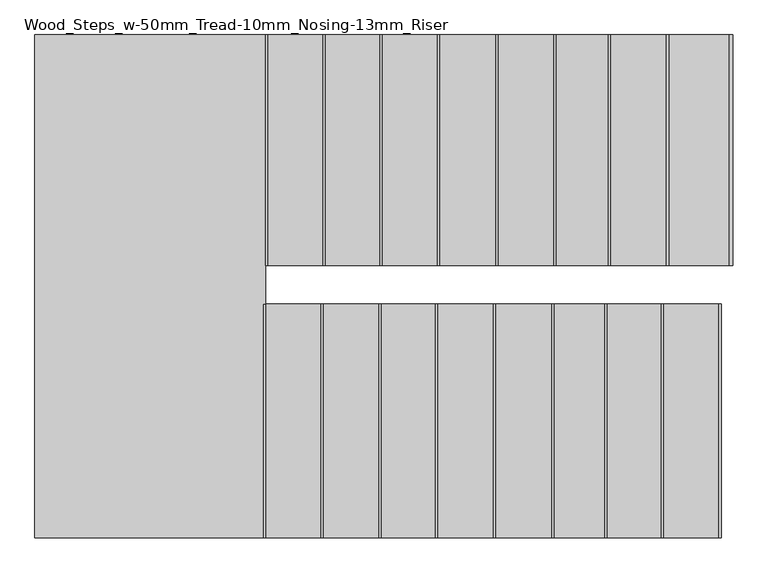
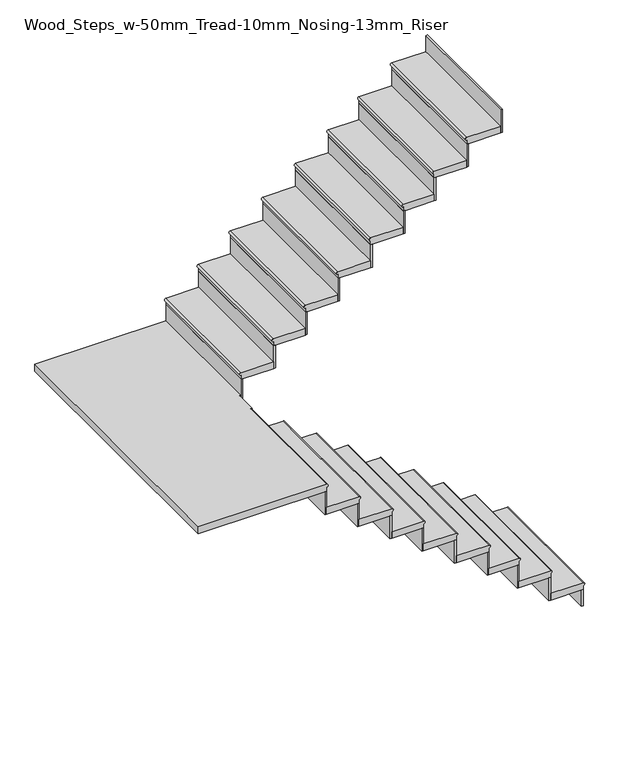
"""IFC4 building model written with IfcOpenShell, lengths in millimetres: stair flight geometry, Wood_Steps_w-50mm_Tread-10mm_Nosing-13mm_Riser."""

from ifc_helpers import new_model, si_unit, frame, origin, place, context, project, spatial, circle_curve, faceted_brep, source, transform, mapped, element, save
from ifc_brep_helpers import plane_surface, cylinder_surface, advanced_brep


def wood_steps_w_50mm_tread_10mm_nosing_13mm_riser_f1b6b8d3(model_context):
    return source(origin(), model_context, "Body", "SolidModel", [
        advanced_brep(
        [(3917.9747157, 6741.6853898, 149.3333333), (3917.9747157, 6741.6853898, 169.3333333), (3917.9747157, 5820.9272041, 169.3333333), (3917.9747157, 5820.9272041, 149.3333333), (3689.3747157, 5820.9272041, 169.3333333), (3689.3747157, 6741.6853898, 169.3333333), (3917.9747157, 5820.9272041, 119.3333333), (3689.3747157, 5820.9272041, 119.3333333), (3689.3747157, 6741.6853898, 119.3333333), (3917.9747157, 6741.6853898, 119.3333333)],
        [
            (0, 1, circle_curve(frame((3917.9747157, 6741.6853898, 159.3333333), z_axis=(0.0, -1.0, 0.0), x_axis=(-1.0, 0.0, 0.0)), 10.0)),
            (1, 2),
            (2, 3, circle_curve(frame((3917.9747157, 5820.9272041, 159.3333333), z_axis=(0.0, 1.0, 0.0), x_axis=(-1.0, 0.0, 0.0)), 10.0)),
            (3, 0),
            (4, 2),
            (1, 5),
            (5, 4),
            (6, 7),
            (7, 8),
            (8, 9),
            (9, 6),
            (4, 7),
            (6, 3),
            (9, 0),
            (8, 5),
        ],
        [
            cylinder_surface(frame((3917.9747157, 6741.6853898, 159.3333333), z_axis=(0.0, 1.0, 0.0), x_axis=(-1.0, 0.0, 0.0)), 10.0),
            plane_surface(frame((3927.9747157, 5820.9272041, 169.3333333), z_axis=(0.0, 0.0, 1.0), x_axis=(1.0, 0.0, 0.0))),
            plane_surface(frame((3927.9747157, 5820.9272041, 119.3333333), z_axis=(0.0, 0.0, -1.0), x_axis=(-1.0, 0.0, 0.0))),
            plane_surface(frame((3689.3747157, 5820.9272041, 169.3333333), z_axis=(0.0, -1.0, 0.0), x_axis=(0.0, 0.0, -1.0))),
            plane_surface(frame((3917.9747157, 5820.9272041, 169.3333333), z_axis=(1.0, 0.0, 0.0), x_axis=(0.0, 0.0, -1.0))),
            plane_surface(frame((3917.9747157, 6741.6853898, 169.3333333), z_axis=(0.0, 1.0, 0.0), x_axis=(0.0, 0.0, -1.0))),
            plane_surface(frame((3689.3747157, 6741.6853898, 169.3333333), z_axis=(-1.0, 0.0, 0.0), x_axis=(0.0, 0.0, -1.0))),
        ],
        [
            (0, [[1, 2, 3, 4]]),
            (1, [[5, -2, 6, 7]]),
            (2, [[8, 9, 10, 11]]),
            (3, [[-5, 12, -8, 13, -3]]),
            (4, [[-11, 14, -4, -13]]),
            (5, [[-6, -1, -14, -10, 15]]),
            (6, [[-7, -15, -9, -12]]),
        ],
    ),
        faceted_brep([(3917.9747157, 6741.6853898, 119.3333333), (3917.9747157, 6741.6853898, 0.0), (3905.4747157, 6741.6853898, 0.0), (3905.4747157, 6741.6853898, 119.3333333), (3917.9747157, 5820.9272041, 119.3333333), (3905.4747157, 5820.9272041, 119.3333333), (3905.4747157, 5820.9272041, 0.0), (3917.9747157, 5820.9272041, 0.0)], [[[0, 1, 2, 3]], [[4, 5, 6, 7]], [[1, 0, 4, 7]], [[2, 1, 7, 6]], [[3, 2, 6, 5]], [[0, 3, 5, 4]]]),
        faceted_brep([(3689.3747157, 6741.6853898, 288.6666667), (3689.3747157, 6741.6853898, 119.3333333), (3676.8747157, 6741.6853898, 119.3333333), (3676.8747157, 6741.6853898, 288.6666667), (3689.3747157, 5820.9272041, 288.6666667), (3676.8747157, 5820.9272041, 288.6666667), (3676.8747157, 5820.9272041, 119.3333333), (3689.3747157, 5820.9272041, 119.3333333)], [[[0, 1, 2, 3]], [[4, 5, 6, 7]], [[1, 0, 4, 7]], [[2, 1, 7, 6]], [[3, 2, 6, 5]], [[0, 3, 5, 4]]]),
        advanced_brep(
        [(3467.1247157, 5820.9272041, 338.6666667), (3689.3747157, 5820.9272041, 338.6666667), (3689.3747157, 6741.6853898, 338.6666667), (3467.1247157, 6741.6853898, 338.6666667), (3689.3747157, 5820.9272041, 288.6666667), (3467.1247157, 5820.9272041, 288.6666667), (3467.1247157, 6741.6853898, 288.6666667), (3689.3747157, 6741.6853898, 288.6666667), (3689.3747157, 5820.9272041, 318.6666667), (3689.3747157, 6741.6853898, 318.6666667)],
        [
            (0, 1),
            (1, 2),
            (2, 3),
            (3, 0),
            (4, 5),
            (5, 6),
            (6, 7),
            (7, 4),
            (0, 5),
            (4, 8),
            (8, 1, circle_curve(frame((3689.3747157, 5820.9272041, 328.6666667), z_axis=(0.0, -1.0, 0.0), x_axis=(-1.0, 0.0, 0.0)), 10.0)),
            (7, 9),
            (9, 8),
            (2, 9, circle_curve(frame((3689.3747157, 6741.6853898, 328.6666667), z_axis=(0.0, 1.0, 0.0), x_axis=(-1.0, 0.0, 0.0)), 10.0)),
            (6, 3),
        ],
        [
            plane_surface(frame((3927.9747157, 5820.9272041, 338.6666667), z_axis=(0.0, 0.0, 1.0), x_axis=(1.0, 0.0, 0.0))),
            plane_surface(frame((3927.9747157, 5820.9272041, 288.6666667), z_axis=(0.0, 0.0, -1.0), x_axis=(-1.0, 0.0, 0.0))),
            plane_surface(frame((3467.1247157, 5820.9272041, 338.6666667), z_axis=(0.0, -1.0, 0.0), x_axis=(0.0, 0.0, -1.0))),
            plane_surface(frame((3689.3747157, 5820.9272041, 338.6666667), z_axis=(1.0, 0.0, 0.0), x_axis=(0.0, 0.0, -1.0))),
            plane_surface(frame((3689.3747157, 6741.6853898, 338.6666667), z_axis=(0.0, 1.0, 0.0), x_axis=(0.0, 0.0, -1.0))),
            plane_surface(frame((3467.1247157, 6741.6853898, 338.6666667), z_axis=(-1.0, 0.0, 0.0), x_axis=(0.0, 0.0, -1.0))),
            cylinder_surface(frame((3689.3747157, 6741.6853898, 328.6666667), z_axis=(0.0, 1.0, 0.0), x_axis=(-1.0, 0.0, 0.0)), 10.0),
        ],
        [
            (0, [[1, 2, 3, 4]]),
            (1, [[5, 6, 7, 8]]),
            (2, [[-1, 9, -5, 10, 11]]),
            (3, [[-8, 12, 13, -10]]),
            (4, [[-3, 14, -12, -7, 15]]),
            (5, [[-4, -15, -6, -9]]),
            (6, [[-14, -2, -11, -13]]),
        ],
    ),
        faceted_brep([(3467.1247157, 6741.6853898, 458.0), (3467.1247157, 6741.6853898, 288.6666667), (3454.6247157, 6741.6853898, 288.6666667), (3454.6247157, 6741.6853898, 458.0), (3467.1247157, 5820.9272041, 458.0), (3454.6247157, 5820.9272041, 458.0), (3454.6247157, 5820.9272041, 288.6666667), (3467.1247157, 5820.9272041, 288.6666667)], [[[0, 1, 2, 3]], [[4, 5, 6, 7]], [[1, 0, 4, 7]], [[2, 1, 7, 6]], [[3, 2, 6, 5]], [[0, 3, 5, 4]]]),
        advanced_brep(
        [(3257.5747157, 5820.9272041, 508.0), (3467.1247157, 5820.9272041, 508.0), (3467.1247157, 6741.6853898, 508.0), (3257.5747157, 6741.6853898, 508.0), (3467.1247157, 5820.9272041, 458.0), (3257.5747157, 5820.9272041, 458.0), (3257.5747157, 6741.6853898, 458.0), (3467.1247157, 6741.6853898, 458.0), (3467.1247157, 5820.9272041, 488.0), (3467.1247157, 6741.6853898, 488.0)],
        [
            (0, 1),
            (1, 2),
            (2, 3),
            (3, 0),
            (4, 5),
            (5, 6),
            (6, 7),
            (7, 4),
            (0, 5),
            (4, 8),
            (8, 1, circle_curve(frame((3467.1247157, 5820.9272041, 498.0), z_axis=(0.0, -1.0, 0.0), x_axis=(-1.0, 0.0, 0.0)), 10.0)),
            (7, 9),
            (9, 8),
            (2, 9, circle_curve(frame((3467.1247157, 6741.6853898, 498.0), z_axis=(0.0, 1.0, 0.0), x_axis=(-1.0, 0.0, 0.0)), 10.0)),
            (6, 3),
        ],
        [
            plane_surface(frame((3927.9747157, 5820.9272041, 508.0), z_axis=(0.0, 0.0, 1.0), x_axis=(1.0, 0.0, 0.0))),
            plane_surface(frame((3927.9747157, 5820.9272041, 458.0), z_axis=(0.0, 0.0, -1.0), x_axis=(-1.0, 0.0, 0.0))),
            plane_surface(frame((3257.5747157, 5820.9272041, 508.0), z_axis=(0.0, -1.0, 0.0), x_axis=(0.0, 0.0, -1.0))),
            plane_surface(frame((3467.1247157, 5820.9272041, 508.0), z_axis=(1.0, 0.0, 0.0), x_axis=(0.0, 0.0, -1.0))),
            plane_surface(frame((3467.1247157, 6741.6853898, 508.0), z_axis=(0.0, 1.0, 0.0), x_axis=(0.0, 0.0, -1.0))),
            plane_surface(frame((3257.5747157, 6741.6853898, 508.0), z_axis=(-1.0, 0.0, 0.0), x_axis=(0.0, 0.0, -1.0))),
            cylinder_surface(frame((3467.1247157, 6741.6853898, 498.0), z_axis=(0.0, 1.0, 0.0), x_axis=(-1.0, 0.0, 0.0)), 10.0),
        ],
        [
            (0, [[1, 2, 3, 4]]),
            (1, [[5, 6, 7, 8]]),
            (2, [[-1, 9, -5, 10, 11]]),
            (3, [[-8, 12, 13, -10]]),
            (4, [[-3, 14, -12, -7, 15]]),
            (5, [[-4, -15, -6, -9]]),
            (6, [[-14, -2, -11, -13]]),
        ],
    ),
        faceted_brep([(3257.5747157, 6741.6853898, 627.3333333), (3257.5747157, 6741.6853898, 458.0), (3245.0747157, 6741.6853898, 458.0), (3245.0747157, 6741.6853898, 627.3333333), (3257.5747157, 5820.9272041, 627.3333333), (3245.0747157, 5820.9272041, 627.3333333), (3245.0747157, 5820.9272041, 458.0), (3257.5747157, 5820.9272041, 458.0)], [[[0, 1, 2, 3]], [[4, 5, 6, 7]], [[1, 0, 4, 7]], [[2, 1, 7, 6]], [[3, 2, 6, 5]], [[0, 3, 5, 4]]]),
        advanced_brep(
        [(3028.9747157, 5820.9272041, 677.3333333), (3257.5747157, 5820.9272041, 677.3333333), (3257.5747157, 6741.6853898, 677.3333333), (3028.9747157, 6741.6853898, 677.3333333), (3257.5747157, 5820.9272041, 627.3333333), (3028.9747157, 5820.9272041, 627.3333333), (3028.9747157, 6741.6853898, 627.3333333), (3257.5747157, 6741.6853898, 627.3333333), (3257.5747157, 5820.9272041, 657.3333333), (3257.5747157, 6741.6853898, 657.3333333)],
        [
            (0, 1),
            (1, 2),
            (2, 3),
            (3, 0),
            (4, 5),
            (5, 6),
            (6, 7),
            (7, 4),
            (0, 5),
            (4, 8),
            (8, 1, circle_curve(frame((3257.5747157, 5820.9272041, 667.3333333), z_axis=(0.0, -1.0, 0.0), x_axis=(-1.0, 0.0, 0.0)), 10.0)),
            (7, 9),
            (9, 8),
            (2, 9, circle_curve(frame((3257.5747157, 6741.6853898, 667.3333333), z_axis=(0.0, 1.0, 0.0), x_axis=(-1.0, 0.0, 0.0)), 10.0)),
            (6, 3),
        ],
        [
            plane_surface(frame((3927.9747157, 5820.9272041, 677.3333333), z_axis=(0.0, 0.0, 1.0), x_axis=(1.0, 0.0, 0.0))),
            plane_surface(frame((3927.9747157, 5820.9272041, 627.3333333), z_axis=(0.0, 0.0, -1.0), x_axis=(-1.0, 0.0, 0.0))),
            plane_surface(frame((3028.9747157, 5820.9272041, 677.3333333), z_axis=(0.0, -1.0, 0.0), x_axis=(0.0, 0.0, -1.0))),
            plane_surface(frame((3257.5747157, 5820.9272041, 677.3333333), z_axis=(1.0, 0.0, 0.0), x_axis=(0.0, 0.0, -1.0))),
            plane_surface(frame((3257.5747157, 6741.6853898, 677.3333333), z_axis=(0.0, 1.0, 0.0), x_axis=(0.0, 0.0, -1.0))),
            plane_surface(frame((3028.9747157, 6741.6853898, 677.3333333), z_axis=(-1.0, 0.0, 0.0), x_axis=(0.0, 0.0, -1.0))),
            cylinder_surface(frame((3257.5747157, 6741.6853898, 667.3333333), z_axis=(0.0, 1.0, 0.0), x_axis=(-1.0, 0.0, 0.0)), 10.0),
        ],
        [
            (0, [[1, 2, 3, 4]]),
            (1, [[5, 6, 7, 8]]),
            (2, [[-1, 9, -5, 10, 11]]),
            (3, [[-8, 12, 13, -10]]),
            (4, [[-3, 14, -12, -7, 15]]),
            (5, [[-4, -15, -6, -9]]),
            (6, [[-14, -2, -11, -13]]),
        ],
    ),
        faceted_brep([(3028.9747157, 6741.6853898, 796.6666667), (3028.9747157, 6741.6853898, 627.3333333), (3016.4747157, 6741.6853898, 627.3333333), (3016.4747157, 6741.6853898, 796.6666667), (3028.9747157, 5820.9272041, 796.6666667), (3016.4747157, 5820.9272041, 796.6666667), (3016.4747157, 5820.9272041, 627.3333333), (3028.9747157, 5820.9272041, 627.3333333)], [[[0, 1, 2, 3]], [[4, 5, 6, 7]], [[1, 0, 4, 7]], [[2, 1, 7, 6]], [[3, 2, 6, 5]], [[0, 3, 5, 4]]]),
        advanced_brep(
        [(2800.3747157, 5820.9272041, 846.6666667), (3028.9747157, 5820.9272041, 846.6666667), (3028.9747157, 6741.6853898, 846.6666667), (2800.3747157, 6741.6853898, 846.6666667), (3028.9747157, 5820.9272041, 796.6666667), (2800.3747157, 5820.9272041, 796.6666667), (2800.3747157, 6741.6853898, 796.6666667), (3028.9747157, 6741.6853898, 796.6666667), (3028.9747157, 5820.9272041, 826.6666667), (3028.9747157, 6741.6853898, 826.6666667)],
        [
            (0, 1),
            (1, 2),
            (2, 3),
            (3, 0),
            (4, 5),
            (5, 6),
            (6, 7),
            (7, 4),
            (0, 5),
            (4, 8),
            (8, 1, circle_curve(frame((3028.9747157, 5820.9272041, 836.6666667), z_axis=(0.0, -1.0, 0.0), x_axis=(-1.0, 0.0, 0.0)), 10.0)),
            (7, 9),
            (9, 8),
            (2, 9, circle_curve(frame((3028.9747157, 6741.6853898, 836.6666667), z_axis=(0.0, 1.0, 0.0), x_axis=(-1.0, 0.0, 0.0)), 10.0)),
            (6, 3),
        ],
        [
            plane_surface(frame((3699.3747157, 5820.9272041, 846.6666667), z_axis=(0.0, 0.0, 1.0), x_axis=(1.0, 0.0, 0.0))),
            plane_surface(frame((3699.3747157, 5820.9272041, 796.6666667), z_axis=(0.0, 0.0, -1.0), x_axis=(-1.0, 0.0, 0.0))),
            plane_surface(frame((2800.3747157, 5820.9272041, 846.6666667), z_axis=(0.0, -1.0, 0.0), x_axis=(0.0, 0.0, -1.0))),
            plane_surface(frame((3028.9747157, 5820.9272041, 846.6666667), z_axis=(1.0, 0.0, 0.0), x_axis=(0.0, 0.0, -1.0))),
            plane_surface(frame((3028.9747157, 6741.6853898, 846.6666667), z_axis=(0.0, 1.0, 0.0), x_axis=(0.0, 0.0, -1.0))),
            plane_surface(frame((2800.3747157, 6741.6853898, 846.6666667), z_axis=(-1.0, 0.0, 0.0), x_axis=(0.0, 0.0, -1.0))),
            cylinder_surface(frame((3028.9747157, 6741.6853898, 836.6666667), z_axis=(0.0, 1.0, 0.0), x_axis=(-1.0, 0.0, 0.0)), 10.0),
        ],
        [
            (0, [[1, 2, 3, 4]]),
            (1, [[5, 6, 7, 8]]),
            (2, [[-1, 9, -5, 10, 11]]),
            (3, [[-8, 12, 13, -10]]),
            (4, [[-3, 14, -12, -7, 15]]),
            (5, [[-4, -15, -6, -9]]),
            (6, [[-14, -2, -11, -13]]),
        ],
    ),
        faceted_brep([(2800.3747157, 6741.6853898, 966.0), (2800.3747157, 6741.6853898, 796.6666667), (2787.8747157, 6741.6853898, 796.6666667), (2787.8747157, 6741.6853898, 966.0), (2800.3747157, 5820.9272041, 966.0), (2787.8747157, 5820.9272041, 966.0), (2787.8747157, 5820.9272041, 796.6666667), (2800.3747157, 5820.9272041, 796.6666667)], [[[0, 1, 2, 3]], [[4, 5, 6, 7]], [[1, 0, 4, 7]], [[2, 1, 7, 6]], [[3, 2, 6, 5]], [[0, 3, 5, 4]]]),
        advanced_brep(
        [(2578.1247157, 5820.9272041, 1016.0), (2800.3747157, 5820.9272041, 1016.0), (2800.3747157, 6741.6853898, 1016.0), (2578.1247157, 6741.6853898, 1016.0), (2800.3747157, 5820.9272041, 966.0), (2578.1247157, 5820.9272041, 966.0), (2578.1247157, 6741.6853898, 966.0), (2800.3747157, 6741.6853898, 966.0), (2800.3747157, 5820.9272041, 996.0), (2800.3747157, 6741.6853898, 996.0)],
        [
            (0, 1),
            (1, 2),
            (2, 3),
            (3, 0),
            (4, 5),
            (5, 6),
            (6, 7),
            (7, 4),
            (0, 5),
            (4, 8),
            (8, 1, circle_curve(frame((2800.3747157, 5820.9272041, 1006.0), z_axis=(0.0, -1.0, 0.0), x_axis=(-1.0, 0.0, 0.0)), 10.0)),
            (7, 9),
            (9, 8),
            (2, 9, circle_curve(frame((2800.3747157, 6741.6853898, 1006.0), z_axis=(0.0, 1.0, 0.0), x_axis=(-1.0, 0.0, 0.0)), 10.0)),
            (6, 3),
        ],
        [
            plane_surface(frame((3927.9747157, 5820.9272041, 1016.0), z_axis=(0.0, 0.0, 1.0), x_axis=(1.0, 0.0, 0.0))),
            plane_surface(frame((3927.9747157, 5820.9272041, 966.0), z_axis=(0.0, 0.0, -1.0), x_axis=(-1.0, 0.0, 0.0))),
            plane_surface(frame((2578.1247157, 5820.9272041, 1016.0), z_axis=(0.0, -1.0, 0.0), x_axis=(0.0, 0.0, -1.0))),
            plane_surface(frame((2800.3747157, 5820.9272041, 1016.0), z_axis=(1.0, 0.0, 0.0), x_axis=(0.0, 0.0, -1.0))),
            plane_surface(frame((2800.3747157, 6741.6853898, 1016.0), z_axis=(0.0, 1.0, 0.0), x_axis=(0.0, 0.0, -1.0))),
            plane_surface(frame((2578.1247157, 6741.6853898, 1016.0), z_axis=(-1.0, 0.0, 0.0), x_axis=(0.0, 0.0, -1.0))),
            cylinder_surface(frame((2800.3747157, 6741.6853898, 1006.0), z_axis=(0.0, 1.0, 0.0), x_axis=(-1.0, 0.0, 0.0)), 10.0),
        ],
        [
            (0, [[1, 2, 3, 4]]),
            (1, [[5, 6, 7, 8]]),
            (2, [[-1, 9, -5, 10, 11]]),
            (3, [[-8, 12, 13, -10]]),
            (4, [[-3, 14, -12, -7, 15]]),
            (5, [[-4, -15, -6, -9]]),
            (6, [[-14, -2, -11, -13]]),
        ],
    ),
        faceted_brep([(2578.1247157, 6741.6853898, 1135.3333333), (2578.1247157, 6741.6853898, 966.0), (2565.6247157, 6741.6853898, 966.0), (2565.6247157, 6741.6853898, 1135.3333333), (2578.1247157, 5820.9272041, 1135.3333333), (2565.6247157, 5820.9272041, 1135.3333333), (2565.6247157, 5820.9272041, 966.0), (2578.1247157, 5820.9272041, 966.0)], [[[0, 1, 2, 3]], [[4, 5, 6, 7]], [[1, 0, 4, 7]], [[2, 1, 7, 6]], [[3, 2, 6, 5]], [[0, 3, 5, 4]]]),
        advanced_brep(
        [(2349.5247157, 5820.9272041, 1185.3333333), (2578.1247157, 5820.9272041, 1185.3333333), (2578.1247157, 6741.6853898, 1185.3333333), (2349.5247157, 6741.6853898, 1185.3333333), (2578.1247157, 5820.9272041, 1135.3333333), (2349.5247157, 5820.9272041, 1135.3333333), (2349.5247157, 6741.6853898, 1135.3333333), (2578.1247157, 6741.6853898, 1135.3333333), (2578.1247157, 5820.9272041, 1165.3333333), (2578.1247157, 6741.6853898, 1165.3333333)],
        [
            (0, 1),
            (1, 2),
            (2, 3),
            (3, 0),
            (4, 5),
            (5, 6),
            (6, 7),
            (7, 4),
            (0, 5),
            (4, 8),
            (8, 1, circle_curve(frame((2578.1247157, 5820.9272041, 1175.3333333), z_axis=(0.0, -1.0, 0.0), x_axis=(-1.0, 0.0, 0.0)), 10.0)),
            (7, 9),
            (9, 8),
            (2, 9, circle_curve(frame((2578.1247157, 6741.6853898, 1175.3333333), z_axis=(0.0, 1.0, 0.0), x_axis=(-1.0, 0.0, 0.0)), 10.0)),
            (6, 3),
        ],
        [
            plane_surface(frame((3927.9747157, 5820.9272041, 1185.3333333), z_axis=(0.0, 0.0, 1.0), x_axis=(1.0, 0.0, 0.0))),
            plane_surface(frame((3927.9747157, 5820.9272041, 1135.3333333), z_axis=(0.0, 0.0, -1.0), x_axis=(-1.0, 0.0, 0.0))),
            plane_surface(frame((2349.5247157, 5820.9272041, 1185.3333333), z_axis=(0.0, -1.0, 0.0), x_axis=(0.0, 0.0, -1.0))),
            plane_surface(frame((2578.1247157, 5820.9272041, 1185.3333333), z_axis=(1.0, 0.0, 0.0), x_axis=(0.0, 0.0, -1.0))),
            plane_surface(frame((2578.1247157, 6741.6853898, 1185.3333333), z_axis=(0.0, 1.0, 0.0), x_axis=(0.0, 0.0, -1.0))),
            plane_surface(frame((2349.5247157, 6741.6853898, 1185.3333333), z_axis=(-1.0, 0.0, 0.0), x_axis=(0.0, 0.0, -1.0))),
            cylinder_surface(frame((2578.1247157, 6741.6853898, 1175.3333333), z_axis=(0.0, 1.0, 0.0), x_axis=(-1.0, 0.0, 0.0)), 10.0),
        ],
        [
            (0, [[1, 2, 3, 4]]),
            (1, [[5, 6, 7, 8]]),
            (2, [[-1, 9, -5, 10, 11]]),
            (3, [[-8, 12, 13, -10]]),
            (4, [[-3, 14, -12, -7, 15]]),
            (5, [[-4, -15, -6, -9]]),
            (6, [[-14, -2, -11, -13]]),
        ],
    ),
        faceted_brep([(2349.5247157, 6741.6853898, 1304.6666667), (2349.5247157, 6741.6853898, 1135.3333333), (2337.0247157, 6741.6853898, 1135.3333333), (2337.0247157, 6741.6853898, 1304.6666667), (2349.5247157, 5820.9272041, 1304.6666667), (2337.0247157, 5820.9272041, 1304.6666667), (2337.0247157, 5820.9272041, 1135.3333333), (2349.5247157, 5820.9272041, 1135.3333333)], [[[0, 1, 2, 3]], [[4, 5, 6, 7]], [[1, 0, 4, 7]], [[2, 1, 7, 6]], [[3, 2, 6, 5]], [[0, 3, 5, 4]]]),
        advanced_brep(
        [(2121.8179225, 5820.9272041, 1354.6666667), (2349.5247157, 5820.9272041, 1354.6666667), (2349.5247157, 6741.6853898, 1354.6666667), (2121.8179225, 6741.6853898, 1354.6666667), (2349.5247157, 5820.9272041, 1304.6666667), (2121.8179225, 5820.9272041, 1304.6666667), (2121.8179225, 6741.6853898, 1304.6666667), (2349.5247157, 6741.6853898, 1304.6666667), (2349.5247157, 5820.9272041, 1334.6666667), (2349.5247157, 6741.6853898, 1334.6666667)],
        [
            (0, 1),
            (1, 2),
            (2, 3),
            (3, 0),
            (4, 5),
            (5, 6),
            (6, 7),
            (7, 4),
            (0, 5),
            (4, 8),
            (8, 1, circle_curve(frame((2349.5247157, 5820.9272041, 1344.6666667), z_axis=(0.0, -1.0, 0.0), x_axis=(-1.0, 0.0, 0.0)), 10.0)),
            (7, 9),
            (9, 8),
            (2, 9, circle_curve(frame((2349.5247157, 6741.6853898, 1344.6666667), z_axis=(0.0, 1.0, 0.0), x_axis=(-1.0, 0.0, 0.0)), 10.0)),
            (6, 3),
        ],
        [
            plane_surface(frame((3927.9747157, 5820.9272041, 1354.6666667), z_axis=(0.0, 0.0, 1.0), x_axis=(1.0, 0.0, 0.0))),
            plane_surface(frame((3927.9747157, 5820.9272041, 1304.6666667), z_axis=(0.0, 0.0, -1.0), x_axis=(-1.0, 0.0, 0.0))),
            plane_surface(frame((2121.8179225, 5820.9272041, 1354.6666667), z_axis=(0.0, -1.0, 0.0), x_axis=(0.0, 0.0, -1.0))),
            plane_surface(frame((2349.5247157, 5820.9272041, 1354.6666667), z_axis=(1.0, 0.0, 0.0), x_axis=(0.0, 0.0, -1.0))),
            plane_surface(frame((2349.5247157, 6741.6853898, 1354.6666667), z_axis=(0.0, 1.0, 0.0), x_axis=(0.0, 0.0, -1.0))),
            plane_surface(frame((2121.8179225, 6741.6853898, 1354.6666667), z_axis=(-1.0, 0.0, 0.0), x_axis=(0.0, 0.0, -1.0))),
            cylinder_surface(frame((2349.5247157, 6741.6853898, 1344.6666667), z_axis=(0.0, 1.0, 0.0), x_axis=(-1.0, 0.0, 0.0)), 10.0),
        ],
        [
            (0, [[1, 2, 3, 4]]),
            (1, [[5, 6, 7, 8]]),
            (2, [[-1, 9, -5, 10, 11]]),
            (3, [[-8, 12, 13, -10]]),
            (4, [[-3, 14, -12, -7, 15]]),
            (5, [[-4, -15, -6, -9]]),
            (6, [[-14, -2, -11, -13]]),
        ],
    ),
        faceted_brep([(2121.8179225, 6741.6853898, 1474.0), (2121.8179225, 6741.6853898, 1304.6666667), (2109.3179225, 6741.6853898, 1304.6666667), (2109.3179225, 6741.6853898, 1474.0), (2121.8179225, 5820.9272041, 1474.0), (2109.3179225, 5820.9272041, 1474.0), (2109.3179225, 5820.9272041, 1304.6666667), (2121.8179225, 5820.9272041, 1304.6666667)], [[[0, 1, 2, 3]], [[4, 5, 6, 7]], [[1, 0, 4, 7]], [[2, 1, 7, 6]], [[3, 2, 6, 5]], [[0, 3, 5, 4]]]),
        advanced_brep(
        [(2141.8179225, 7802.1353898, 1524.0), (1223.7679225, 7802.1353898, 1524.0), (1223.7679225, 5820.9272041, 1524.0), (2121.8179225, 5820.9272041, 1524.0), (2121.8179225, 6741.6853898, 1524.0), (2131.8179225, 6741.6853898, 1524.0), (2131.8179225, 6894.0853898, 1524.0), (2141.8179225, 6894.0853898, 1524.0), (1223.7679225, 7802.1353898, 1474.0), (2141.8179225, 7802.1353898, 1474.0), (2141.8179225, 6894.0853898, 1474.0), (2131.8179225, 6894.0853898, 1474.0), (2131.8179225, 6741.6853898, 1474.0), (2121.8179225, 6741.6853898, 1474.0), (2121.8179225, 5820.9272041, 1474.0), (1223.7679225, 5820.9272041, 1474.0), (2121.8179225, 5820.9272041, 1504.0), (2121.8179225, 6741.6853898, 1504.0), (2131.8179225, 6741.6853898, 1514.0)],
        [
            (0, 1),
            (1, 2),
            (2, 3),
            (3, 4),
            (4, 5),
            (5, 6),
            (6, 7),
            (7, 0),
            (8, 9),
            (9, 10),
            (10, 11),
            (11, 12),
            (12, 13),
            (13, 14),
            (14, 15),
            (15, 8),
            (0, 9),
            (8, 1),
            (15, 2),
            (14, 16),
            (16, 3, circle_curve(frame((2121.8179225, 5820.9272041, 1514.0), z_axis=(0.0, -1.0, 0.0), x_axis=(-1.0, 0.0, 0.0)), 10.0)),
            (13, 17),
            (17, 16),
            (4, 18, circle_curve(frame((2121.8179225, 6741.6853898, 1514.0), z_axis=(0.0, 1.0, 0.0), x_axis=(-1.0, 0.0, 0.0)), 10.0)),
            (18, 5),
            (12, 18),
            (18, 17, circle_curve(frame((2121.8179225, 6741.6853898, 1514.0), z_axis=(0.0, 1.0, 0.0), x_axis=(-1.0, 0.0, 0.0)), 10.0)),
            (11, 6),
            (10, 7),
        ],
        [
            plane_surface(frame((1223.7679225, 7802.1353898, 1524.0), z_axis=(0.0, 0.0, 1.0), x_axis=(-1.0, 0.0, 0.0))),
            plane_surface(frame((1223.7679225, 7802.1353898, 1474.0), z_axis=(0.0, 0.0, -1.0), x_axis=(1.0, 0.0, 0.0))),
            plane_surface(frame((2141.8179225, 7802.1353898, 1524.0), z_axis=(0.0, 1.0, 0.0), x_axis=(0.0, 0.0, -1.0))),
            plane_surface(frame((1223.7679225, 7802.1353898, 1524.0), z_axis=(-1.0, 0.0, 0.0), x_axis=(0.0, 0.0, -1.0))),
            plane_surface(frame((1223.7679225, 5820.9272041, 1524.0), z_axis=(0.0, -1.0, 0.0), x_axis=(0.0, 0.0, -1.0))),
            plane_surface(frame((2121.8179225, 5820.9272041, 1524.0), z_axis=(1.0, 0.0, 0.0), x_axis=(0.0, 0.0, -1.0))),
            plane_surface(frame((2121.8179225, 6741.6853898, 1524.0), z_axis=(0.0, -1.0, 0.0), x_axis=(0.0, 0.0, -1.0))),
            plane_surface(frame((2131.8179225, 6741.6853898, 1524.0), z_axis=(1.0, 0.0, 0.0), x_axis=(0.0, 0.0, -1.0))),
            plane_surface(frame((2131.8179225, 6894.0853898, 1524.0), z_axis=(0.0, -1.0, 0.0), x_axis=(0.0, 0.0, -1.0))),
            plane_surface(frame((2141.8179225, 6894.0853898, 1524.0), z_axis=(1.0, 0.0, 0.0), x_axis=(0.0, 0.0, -1.0))),
            cylinder_surface(frame((2121.8179225, 6741.6853898, 1514.0), z_axis=(0.0, 1.0, 0.0), x_axis=(-1.0, 0.0, 0.0)), 10.0),
        ],
        [
            (0, [[1, 2, 3, 4, 5, 6, 7, 8]]),
            (1, [[9, 10, 11, 12, 13, 14, 15, 16]]),
            (2, [[-1, 17, -9, 18]]),
            (3, [[-2, -18, -16, 19]]),
            (4, [[-3, -19, -15, 20, 21]]),
            (5, [[-14, 22, 23, -20]]),
            (6, [[-5, 24, 25]]),
            (6, [[-13, 26, 27, -22]]),
            (7, [[-6, -25, -26, -12, 28]]),
            (8, [[-7, -28, -11, 29]]),
            (9, [[-8, -29, -10, -17]]),
            (10, [[-21, -23, -27, -24, -4]]),
        ],
    ),
        faceted_brep([(2141.8179225, 6894.0853898, 1643.3333333), (2141.8179225, 6894.0853898, 1474.0), (2154.3179225, 6894.0853898, 1474.0), (2154.3179225, 6894.0853898, 1643.3333333), (2141.8179225, 7802.1353898, 1643.3333333), (2154.3179225, 7802.1353898, 1643.3333333), (2154.3179225, 7802.1353898, 1474.0), (2141.8179225, 7802.1353898, 1474.0)], [[[0, 1, 2, 3]], [[4, 5, 6, 7]], [[1, 0, 4, 7]], [[2, 1, 7, 6]], [[3, 2, 6, 5]], [[0, 3, 5, 4]]]),
        advanced_brep(
        [(2369.5247157, 7802.1353898, 1693.3333333), (2141.8179225, 7802.1353898, 1693.3333333), (2141.8179225, 6894.0853898, 1693.3333333), (2369.5247157, 6894.0853898, 1693.3333333), (2141.8179225, 7802.1353898, 1643.3333333), (2369.5247157, 7802.1353898, 1643.3333333), (2369.5247157, 6894.0853898, 1643.3333333), (2141.8179225, 6894.0853898, 1643.3333333), (2141.8179225, 7802.1353898, 1673.3333333), (2141.8179225, 6894.0853898, 1673.3333333)],
        [
            (0, 1),
            (1, 2),
            (2, 3),
            (3, 0),
            (4, 5),
            (5, 6),
            (6, 7),
            (7, 4),
            (0, 5),
            (4, 8),
            (8, 1, circle_curve(frame((2141.8179225, 7802.1353898, 1683.3333333), z_axis=(0.0, 1.0, 0.0), x_axis=(1.0, 0.0, 0.0)), 10.0)),
            (7, 9),
            (9, 8),
            (2, 9, circle_curve(frame((2141.8179225, 6894.0853898, 1683.3333333), z_axis=(0.0, -1.0, 0.0), x_axis=(1.0, 0.0, 0.0)), 10.0)),
            (6, 3),
        ],
        [
            plane_surface(frame((1223.7679225, 7802.1353898, 1693.3333333), z_axis=(0.0, 0.0, 1.0), x_axis=(-1.0, 0.0, 0.0))),
            plane_surface(frame((1223.7679225, 7802.1353898, 1643.3333333), z_axis=(0.0, 0.0, -1.0), x_axis=(1.0, 0.0, 0.0))),
            plane_surface(frame((2369.5247157, 7802.1353898, 1693.3333333), z_axis=(0.0, 1.0, 0.0), x_axis=(0.0, 0.0, -1.0))),
            plane_surface(frame((2141.8179225, 7802.1353898, 1693.3333333), z_axis=(-1.0, 0.0, 0.0), x_axis=(0.0, 0.0, -1.0))),
            plane_surface(frame((2141.8179225, 6894.0853898, 1693.3333333), z_axis=(0.0, -1.0, 0.0), x_axis=(0.0, 0.0, -1.0))),
            plane_surface(frame((2369.5247157, 6894.0853898, 1693.3333333), z_axis=(1.0, 0.0, 0.0), x_axis=(0.0, 0.0, -1.0))),
            cylinder_surface(frame((2141.8179225, 6894.0853898, 1683.3333333), z_axis=(0.0, -1.0, 0.0), x_axis=(1.0, 0.0, 0.0)), 10.0),
        ],
        [
            (0, [[1, 2, 3, 4]]),
            (1, [[5, 6, 7, 8]]),
            (2, [[-1, 9, -5, 10, 11]]),
            (3, [[-8, 12, 13, -10]]),
            (4, [[-3, 14, -12, -7, 15]]),
            (5, [[-4, -15, -6, -9]]),
            (6, [[-14, -2, -11, -13]]),
        ],
    ),
        faceted_brep([(2369.5247157, 6894.0853898, 1812.6666667), (2369.5247157, 6894.0853898, 1643.3333333), (2382.0247157, 6894.0853898, 1643.3333333), (2382.0247157, 6894.0853898, 1812.6666667), (2369.5247157, 7802.1353898, 1812.6666667), (2382.0247157, 7802.1353898, 1812.6666667), (2382.0247157, 7802.1353898, 1643.3333333), (2369.5247157, 7802.1353898, 1643.3333333)], [[[0, 1, 2, 3]], [[4, 5, 6, 7]], [[1, 0, 4, 7]], [[2, 1, 7, 6]], [[3, 2, 6, 5]], [[0, 3, 5, 4]]]),
        advanced_brep(
        [(2592.6679225, 7802.1353898, 1862.6666667), (2369.5247157, 7802.1353898, 1862.6666667), (2369.5247157, 6894.0853898, 1862.6666667), (2592.6679225, 6894.0853898, 1862.6666667), (2369.5247157, 7802.1353898, 1812.6666667), (2592.6679225, 7802.1353898, 1812.6666667), (2592.6679225, 6894.0853898, 1812.6666667), (2369.5247157, 6894.0853898, 1812.6666667), (2369.5247157, 7802.1353898, 1842.6666667), (2369.5247157, 6894.0853898, 1842.6666667)],
        [
            (0, 1),
            (1, 2),
            (2, 3),
            (3, 0),
            (4, 5),
            (5, 6),
            (6, 7),
            (7, 4),
            (0, 5),
            (4, 8),
            (8, 1, circle_curve(frame((2369.5247157, 7802.1353898, 1852.6666667), z_axis=(0.0, 1.0, 0.0), x_axis=(1.0, 0.0, 0.0)), 10.0)),
            (7, 9),
            (9, 8),
            (2, 9, circle_curve(frame((2369.5247157, 6894.0853898, 1852.6666667), z_axis=(0.0, -1.0, 0.0), x_axis=(1.0, 0.0, 0.0)), 10.0)),
            (6, 3),
        ],
        [
            plane_surface(frame((1223.7679225, 7802.1353898, 1862.6666667), z_axis=(0.0, 0.0, 1.0), x_axis=(-1.0, 0.0, 0.0))),
            plane_surface(frame((1223.7679225, 7802.1353898, 1812.6666667), z_axis=(0.0, 0.0, -1.0), x_axis=(1.0, 0.0, 0.0))),
            plane_surface(frame((2592.6679225, 7802.1353898, 1862.6666667), z_axis=(0.0, 1.0, 0.0), x_axis=(0.0, 0.0, -1.0))),
            plane_surface(frame((2369.5247157, 7802.1353898, 1862.6666667), z_axis=(-1.0, 0.0, 0.0), x_axis=(0.0, 0.0, -1.0))),
            plane_surface(frame((2369.5247157, 6894.0853898, 1862.6666667), z_axis=(0.0, -1.0, 0.0), x_axis=(0.0, 0.0, -1.0))),
            plane_surface(frame((2592.6679225, 6894.0853898, 1862.6666667), z_axis=(1.0, 0.0, 0.0), x_axis=(0.0, 0.0, -1.0))),
            cylinder_surface(frame((2369.5247157, 6894.0853898, 1852.6666667), z_axis=(0.0, -1.0, 0.0), x_axis=(1.0, 0.0, 0.0)), 10.0),
        ],
        [
            (0, [[1, 2, 3, 4]]),
            (1, [[5, 6, 7, 8]]),
            (2, [[-1, 9, -5, 10, 11]]),
            (3, [[-8, 12, 13, -10]]),
            (4, [[-3, 14, -12, -7, 15]]),
            (5, [[-4, -15, -6, -9]]),
            (6, [[-14, -2, -11, -13]]),
        ],
    ),
        faceted_brep([(2592.6679225, 6894.0853898, 1982.0), (2592.6679225, 6894.0853898, 1812.6666667), (2605.1679225, 6894.0853898, 1812.6666667), (2605.1679225, 6894.0853898, 1982.0), (2592.6679225, 7802.1353898, 1982.0), (2605.1679225, 7802.1353898, 1982.0), (2605.1679225, 7802.1353898, 1812.6666667), (2592.6679225, 7802.1353898, 1812.6666667)], [[[0, 1, 2, 3]], [[4, 5, 6, 7]], [[1, 0, 4, 7]], [[2, 1, 7, 6]], [[3, 2, 6, 5]], [[0, 3, 5, 4]]]),
        advanced_brep(
        [(2820.3747157, 7802.1353898, 2032.0), (2592.6679225, 7802.1353898, 2032.0), (2592.6679225, 6894.0853898, 2032.0), (2820.3747157, 6894.0853898, 2032.0), (2592.6679225, 7802.1353898, 1982.0), (2820.3747157, 7802.1353898, 1982.0), (2820.3747157, 6894.0853898, 1982.0), (2592.6679225, 6894.0853898, 1982.0), (2592.6679225, 7802.1353898, 2012.0), (2592.6679225, 6894.0853898, 2012.0)],
        [
            (0, 1),
            (1, 2),
            (2, 3),
            (3, 0),
            (4, 5),
            (5, 6),
            (6, 7),
            (7, 4),
            (0, 5),
            (4, 8),
            (8, 1, circle_curve(frame((2592.6679225, 7802.1353898, 2022.0), z_axis=(0.0, 1.0, 0.0), x_axis=(1.0, 0.0, 0.0)), 10.0)),
            (7, 9),
            (9, 8),
            (2, 9, circle_curve(frame((2592.6679225, 6894.0853898, 2022.0), z_axis=(0.0, -1.0, 0.0), x_axis=(1.0, 0.0, 0.0)), 10.0)),
            (6, 3),
        ],
        [
            plane_surface(frame((1223.7679225, 7802.1353898, 2032.0), z_axis=(0.0, 0.0, 1.0), x_axis=(-1.0, 0.0, 0.0))),
            plane_surface(frame((1223.7679225, 7802.1353898, 1982.0), z_axis=(0.0, 0.0, -1.0), x_axis=(1.0, 0.0, 0.0))),
            plane_surface(frame((2820.3747157, 7802.1353898, 2032.0), z_axis=(0.0, 1.0, 0.0), x_axis=(0.0, 0.0, -1.0))),
            plane_surface(frame((2592.6679225, 7802.1353898, 2032.0), z_axis=(-1.0, 0.0, 0.0), x_axis=(0.0, 0.0, -1.0))),
            plane_surface(frame((2592.6679225, 6894.0853898, 2032.0), z_axis=(0.0, -1.0, 0.0), x_axis=(0.0, 0.0, -1.0))),
            plane_surface(frame((2820.3747157, 6894.0853898, 2032.0), z_axis=(1.0, 0.0, 0.0), x_axis=(0.0, 0.0, -1.0))),
            cylinder_surface(frame((2592.6679225, 6894.0853898, 2022.0), z_axis=(0.0, -1.0, 0.0), x_axis=(1.0, 0.0, 0.0)), 10.0),
        ],
        [
            (0, [[1, 2, 3, 4]]),
            (1, [[5, 6, 7, 8]]),
            (2, [[-1, 9, -5, 10, 11]]),
            (3, [[-8, 12, 13, -10]]),
            (4, [[-3, 14, -12, -7, 15]]),
            (5, [[-4, -15, -6, -9]]),
            (6, [[-14, -2, -11, -13]]),
        ],
    ),
        faceted_brep([(2820.3747157, 6894.0853898, 2151.3333333), (2820.3747157, 6894.0853898, 1982.0), (2832.8747157, 6894.0853898, 1982.0), (2832.8747157, 6894.0853898, 2151.3333333), (2820.3747157, 7802.1353898, 2151.3333333), (2832.8747157, 7802.1353898, 2151.3333333), (2832.8747157, 7802.1353898, 1982.0), (2820.3747157, 7802.1353898, 1982.0)], [[[0, 1, 2, 3]], [[4, 5, 6, 7]], [[1, 0, 4, 7]], [[2, 1, 7, 6]], [[3, 2, 6, 5]], [[0, 3, 5, 4]]]),
        advanced_brep(
        [(3048.9747157, 7802.1353898, 2201.3333333), (2820.3747157, 7802.1353898, 2201.3333333), (2820.3747157, 6894.0853898, 2201.3333333), (3048.9747157, 6894.0853898, 2201.3333333), (2820.3747157, 7802.1353898, 2151.3333333), (3048.9747157, 7802.1353898, 2151.3333333), (3048.9747157, 6894.0853898, 2151.3333333), (2820.3747157, 6894.0853898, 2151.3333333), (2820.3747157, 7802.1353898, 2181.3333333), (2820.3747157, 6894.0853898, 2181.3333333)],
        [
            (0, 1),
            (1, 2),
            (2, 3),
            (3, 0),
            (4, 5),
            (5, 6),
            (6, 7),
            (7, 4),
            (0, 5),
            (4, 8),
            (8, 1, circle_curve(frame((2820.3747157, 7802.1353898, 2191.3333333), z_axis=(0.0, 1.0, 0.0), x_axis=(1.0, 0.0, 0.0)), 10.0)),
            (7, 9),
            (9, 8),
            (2, 9, circle_curve(frame((2820.3747157, 6894.0853898, 2191.3333333), z_axis=(0.0, -1.0, 0.0), x_axis=(1.0, 0.0, 0.0)), 10.0)),
            (6, 3),
        ],
        [
            plane_surface(frame((1223.7679225, 7802.1353898, 2201.3333333), z_axis=(0.0, 0.0, 1.0), x_axis=(-1.0, 0.0, 0.0))),
            plane_surface(frame((1223.7679225, 7802.1353898, 2151.3333333), z_axis=(0.0, 0.0, -1.0), x_axis=(1.0, 0.0, 0.0))),
            plane_surface(frame((3048.9747157, 7802.1353898, 2201.3333333), z_axis=(0.0, 1.0, 0.0), x_axis=(0.0, 0.0, -1.0))),
            plane_surface(frame((2820.3747157, 7802.1353898, 2201.3333333), z_axis=(-1.0, 0.0, 0.0), x_axis=(0.0, 0.0, -1.0))),
            plane_surface(frame((2820.3747157, 6894.0853898, 2201.3333333), z_axis=(0.0, -1.0, 0.0), x_axis=(0.0, 0.0, -1.0))),
            plane_surface(frame((3048.9747157, 6894.0853898, 2201.3333333), z_axis=(1.0, 0.0, 0.0), x_axis=(0.0, 0.0, -1.0))),
            cylinder_surface(frame((2820.3747157, 6894.0853898, 2191.3333333), z_axis=(0.0, -1.0, 0.0), x_axis=(1.0, 0.0, 0.0)), 10.0),
        ],
        [
            (0, [[1, 2, 3, 4]]),
            (1, [[5, 6, 7, 8]]),
            (2, [[-1, 9, -5, 10, 11]]),
            (3, [[-8, 12, 13, -10]]),
            (4, [[-3, 14, -12, -7, 15]]),
            (5, [[-4, -15, -6, -9]]),
            (6, [[-14, -2, -11, -13]]),
        ],
    ),
        faceted_brep([(3048.9747157, 6894.0853898, 2320.6666667), (3048.9747157, 6894.0853898, 2151.3333333), (3061.4747157, 6894.0853898, 2151.3333333), (3061.4747157, 6894.0853898, 2320.6666667), (3048.9747157, 7802.1353898, 2320.6666667), (3061.4747157, 7802.1353898, 2320.6666667), (3061.4747157, 7802.1353898, 2151.3333333), (3048.9747157, 7802.1353898, 2151.3333333)], [[[0, 1, 2, 3]], [[4, 5, 6, 7]], [[1, 0, 4, 7]], [[2, 1, 7, 6]], [[3, 2, 6, 5]], [[0, 3, 5, 4]]]),
        advanced_brep(
        [(3277.5747157, 7802.1353898, 2370.6666667), (3048.9747157, 7802.1353898, 2370.6666667), (3048.9747157, 6894.0853898, 2370.6666667), (3277.5747157, 6894.0853898, 2370.6666667), (3048.9747157, 7802.1353898, 2320.6666667), (3277.5747157, 7802.1353898, 2320.6666667), (3277.5747157, 6894.0853898, 2320.6666667), (3048.9747157, 6894.0853898, 2320.6666667), (3048.9747157, 7802.1353898, 2350.6666667), (3048.9747157, 6894.0853898, 2350.6666667)],
        [
            (0, 1),
            (1, 2),
            (2, 3),
            (3, 0),
            (4, 5),
            (5, 6),
            (6, 7),
            (7, 4),
            (0, 5),
            (4, 8),
            (8, 1, circle_curve(frame((3048.9747157, 7802.1353898, 2360.6666667), z_axis=(0.0, 1.0, 0.0), x_axis=(1.0, 0.0, 0.0)), 10.0)),
            (7, 9),
            (9, 8),
            (2, 9, circle_curve(frame((3048.9747157, 6894.0853898, 2360.6666667), z_axis=(0.0, -1.0, 0.0), x_axis=(1.0, 0.0, 0.0)), 10.0)),
            (6, 3),
        ],
        [
            plane_surface(frame((1452.3679225, 7802.1353898, 2370.6666667), z_axis=(0.0, 0.0, 1.0), x_axis=(-1.0, 0.0, 0.0))),
            plane_surface(frame((1452.3679225, 7802.1353898, 2320.6666667), z_axis=(0.0, 0.0, -1.0), x_axis=(1.0, 0.0, 0.0))),
            plane_surface(frame((3277.5747157, 7802.1353898, 2370.6666667), z_axis=(0.0, 1.0, 0.0), x_axis=(0.0, 0.0, -1.0))),
            plane_surface(frame((3048.9747157, 7802.1353898, 2370.6666667), z_axis=(-1.0, 0.0, 0.0), x_axis=(0.0, 0.0, -1.0))),
            plane_surface(frame((3048.9747157, 6894.0853898, 2370.6666667), z_axis=(0.0, -1.0, 0.0), x_axis=(0.0, 0.0, -1.0))),
            plane_surface(frame((3277.5747157, 6894.0853898, 2370.6666667), z_axis=(1.0, 0.0, 0.0), x_axis=(0.0, 0.0, -1.0))),
            cylinder_surface(frame((3048.9747157, 6894.0853898, 2360.6666667), z_axis=(0.0, -1.0, 0.0), x_axis=(1.0, 0.0, 0.0)), 10.0),
        ],
        [
            (0, [[1, 2, 3, 4]]),
            (1, [[5, 6, 7, 8]]),
            (2, [[-1, 9, -5, 10, 11]]),
            (3, [[-8, 12, 13, -10]]),
            (4, [[-3, 14, -12, -7, 15]]),
            (5, [[-4, -15, -6, -9]]),
            (6, [[-14, -2, -11, -13]]),
        ],
    ),
        faceted_brep([(3277.5747157, 6894.0853898, 2490.0), (3277.5747157, 6894.0853898, 2320.6666667), (3290.0747157, 6894.0853898, 2320.6666667), (3290.0747157, 6894.0853898, 2490.0), (3277.5747157, 7802.1353898, 2490.0), (3290.0747157, 7802.1353898, 2490.0), (3290.0747157, 7802.1353898, 2320.6666667), (3277.5747157, 7802.1353898, 2320.6666667)], [[[0, 1, 2, 3]], [[4, 5, 6, 7]], [[1, 0, 4, 7]], [[2, 1, 7, 6]], [[3, 2, 6, 5]], [[0, 3, 5, 4]]]),
        advanced_brep(
        [(3493.4747157, 7802.1353898, 2540.0), (3277.5747157, 7802.1353898, 2540.0), (3277.5747157, 6894.0853898, 2540.0), (3493.4747157, 6894.0853898, 2540.0), (3277.5747157, 7802.1353898, 2490.0), (3493.4747157, 7802.1353898, 2490.0), (3493.4747157, 6894.0853898, 2490.0), (3277.5747157, 6894.0853898, 2490.0), (3277.5747157, 7802.1353898, 2520.0), (3277.5747157, 6894.0853898, 2520.0)],
        [
            (0, 1),
            (1, 2),
            (2, 3),
            (3, 0),
            (4, 5),
            (5, 6),
            (6, 7),
            (7, 4),
            (0, 5),
            (4, 8),
            (8, 1, circle_curve(frame((3277.5747157, 7802.1353898, 2530.0), z_axis=(0.0, 1.0, 0.0), x_axis=(1.0, 0.0, 0.0)), 10.0)),
            (7, 9),
            (9, 8),
            (2, 9, circle_curve(frame((3277.5747157, 6894.0853898, 2530.0), z_axis=(0.0, -1.0, 0.0), x_axis=(1.0, 0.0, 0.0)), 10.0)),
            (6, 3),
        ],
        [
            plane_surface(frame((1223.7679225, 7802.1353898, 2540.0), z_axis=(0.0, 0.0, 1.0), x_axis=(-1.0, 0.0, 0.0))),
            plane_surface(frame((1223.7679225, 7802.1353898, 2490.0), z_axis=(0.0, 0.0, -1.0), x_axis=(1.0, 0.0, 0.0))),
            plane_surface(frame((3493.4747157, 7802.1353898, 2540.0), z_axis=(0.0, 1.0, 0.0), x_axis=(0.0, 0.0, -1.0))),
            plane_surface(frame((3277.5747157, 7802.1353898, 2540.0), z_axis=(-1.0, 0.0, 0.0), x_axis=(0.0, 0.0, -1.0))),
            plane_surface(frame((3277.5747157, 6894.0853898, 2540.0), z_axis=(0.0, -1.0, 0.0), x_axis=(0.0, 0.0, -1.0))),
            plane_surface(frame((3493.4747157, 6894.0853898, 2540.0), z_axis=(1.0, 0.0, 0.0), x_axis=(0.0, 0.0, -1.0))),
            cylinder_surface(frame((3277.5747157, 6894.0853898, 2530.0), z_axis=(0.0, -1.0, 0.0), x_axis=(1.0, 0.0, 0.0)), 10.0),
        ],
        [
            (0, [[1, 2, 3, 4]]),
            (1, [[5, 6, 7, 8]]),
            (2, [[-1, 9, -5, 10, 11]]),
            (3, [[-8, 12, 13, -10]]),
            (4, [[-3, 14, -12, -7, 15]]),
            (5, [[-4, -15, -6, -9]]),
            (6, [[-14, -2, -11, -13]]),
        ],
    ),
        faceted_brep([(3493.4747157, 6894.0853898, 2659.3333333), (3493.4747157, 6894.0853898, 2490.0), (3505.9747157, 6894.0853898, 2490.0), (3505.9747157, 6894.0853898, 2659.3333333), (3493.4747157, 7802.1353898, 2659.3333333), (3505.9747157, 7802.1353898, 2659.3333333), (3505.9747157, 7802.1353898, 2490.0), (3493.4747157, 7802.1353898, 2490.0)], [[[0, 1, 2, 3]], [[4, 5, 6, 7]], [[1, 0, 4, 7]], [[2, 1, 7, 6]], [[3, 2, 6, 5]], [[0, 3, 5, 4]]]),
        advanced_brep(
        [(3722.0747157, 7802.1353898, 2709.3333333), (3493.4747157, 7802.1353898, 2709.3333333), (3493.4747157, 6894.0853898, 2709.3333333), (3722.0747157, 6894.0853898, 2709.3333333), (3493.4747157, 7802.1353898, 2659.3333333), (3722.0747157, 7802.1353898, 2659.3333333), (3722.0747157, 6894.0853898, 2659.3333333), (3493.4747157, 6894.0853898, 2659.3333333), (3493.4747157, 7802.1353898, 2689.3333333), (3493.4747157, 6894.0853898, 2689.3333333)],
        [
            (0, 1),
            (1, 2),
            (2, 3),
            (3, 0),
            (4, 5),
            (5, 6),
            (6, 7),
            (7, 4),
            (0, 5),
            (4, 8),
            (8, 1, circle_curve(frame((3493.4747157, 7802.1353898, 2699.3333333), z_axis=(0.0, 1.0, 0.0), x_axis=(1.0, 0.0, 0.0)), 10.0)),
            (7, 9),
            (9, 8),
            (2, 9, circle_curve(frame((3493.4747157, 6894.0853898, 2699.3333333), z_axis=(0.0, -1.0, 0.0), x_axis=(1.0, 0.0, 0.0)), 10.0)),
            (6, 3),
        ],
        [
            plane_surface(frame((1223.7679225, 7802.1353898, 2709.3333333), z_axis=(0.0, 0.0, 1.0), x_axis=(-1.0, 0.0, 0.0))),
            plane_surface(frame((1223.7679225, 7802.1353898, 2659.3333333), z_axis=(0.0, 0.0, -1.0), x_axis=(1.0, 0.0, 0.0))),
            plane_surface(frame((3722.0747157, 7802.1353898, 2709.3333333), z_axis=(0.0, 1.0, 0.0), x_axis=(0.0, 0.0, -1.0))),
            plane_surface(frame((3493.4747157, 7802.1353898, 2709.3333333), z_axis=(-1.0, 0.0, 0.0), x_axis=(0.0, 0.0, -1.0))),
            plane_surface(frame((3493.4747157, 6894.0853898, 2709.3333333), z_axis=(0.0, -1.0, 0.0), x_axis=(0.0, 0.0, -1.0))),
            plane_surface(frame((3722.0747157, 6894.0853898, 2709.3333333), z_axis=(1.0, 0.0, 0.0), x_axis=(0.0, 0.0, -1.0))),
            cylinder_surface(frame((3493.4747157, 6894.0853898, 2699.3333333), z_axis=(0.0, -1.0, 0.0), x_axis=(1.0, 0.0, 0.0)), 10.0),
        ],
        [
            (0, [[1, 2, 3, 4]]),
            (1, [[5, 6, 7, 8]]),
            (2, [[-1, 9, -5, 10, 11]]),
            (3, [[-8, 12, 13, -10]]),
            (4, [[-3, 14, -12, -7, 15]]),
            (5, [[-4, -15, -6, -9]]),
            (6, [[-14, -2, -11, -13]]),
        ],
    ),
        faceted_brep([(3722.0747157, 6894.0853898, 2828.6666667), (3722.0747157, 6894.0853898, 2659.3333333), (3734.5747157, 6894.0853898, 2659.3333333), (3734.5747157, 6894.0853898, 2828.6666667), (3722.0747157, 7802.1353898, 2828.6666667), (3734.5747157, 7802.1353898, 2828.6666667), (3734.5747157, 7802.1353898, 2659.3333333), (3722.0747157, 7802.1353898, 2659.3333333)], [[[0, 1, 2, 3]], [[4, 5, 6, 7]], [[1, 0, 4, 7]], [[2, 1, 7, 6]], [[3, 2, 6, 5]], [[0, 3, 5, 4]]]),
        faceted_brep([(3959.8187157, 6894.0853898, 2998.0), (3959.8187157, 6894.0853898, 2828.6666667), (3972.3187157, 6894.0853898, 2828.6666667), (3972.3187157, 6894.0853898, 2998.0), (3959.8187157, 7802.1353898, 2998.0), (3972.3187157, 7802.1353898, 2998.0), (3972.3187157, 7802.1353898, 2828.6666667), (3959.8187157, 7802.1353898, 2828.6666667)], [[[0, 1, 2, 3]], [[4, 5, 6, 7]], [[1, 0, 4, 7]], [[2, 1, 7, 6]], [[3, 2, 6, 5]], [[0, 3, 5, 4]]]),
        advanced_brep(
        [(3959.8187157, 7802.1353898, 2878.6666667), (3722.0747157, 7802.1353898, 2878.6666667), (3722.0747157, 6894.0853898, 2878.6666667), (3959.8187157, 6894.0853898, 2878.6666667), (3722.0747157, 7802.1353898, 2828.6666667), (3959.8187157, 7802.1353898, 2828.6666667), (3959.8187157, 6894.0853898, 2828.6666667), (3722.0747157, 6894.0853898, 2828.6666667), (3722.0747157, 7802.1353898, 2858.6666667), (3722.0747157, 6894.0853898, 2858.6666667)],
        [
            (0, 1),
            (1, 2),
            (2, 3),
            (3, 0),
            (4, 5),
            (5, 6),
            (6, 7),
            (7, 4),
            (0, 5),
            (4, 8),
            (8, 1, circle_curve(frame((3722.0747157, 7802.1353898, 2868.6666667), z_axis=(0.0, 1.0, 0.0), x_axis=(1.0, 0.0, 0.0)), 10.0)),
            (7, 9),
            (9, 8),
            (2, 9, circle_curve(frame((3722.0747157, 6894.0853898, 2868.6666667), z_axis=(0.0, -1.0, 0.0), x_axis=(1.0, 0.0, 0.0)), 10.0)),
            (6, 3),
        ],
        [
            plane_surface(frame((1223.7679225, 7802.1353898, 2878.6666667), z_axis=(0.0, 0.0, 1.0), x_axis=(-1.0, 0.0, 0.0))),
            plane_surface(frame((1223.7679225, 7802.1353898, 2828.6666667), z_axis=(0.0, 0.0, -1.0), x_axis=(1.0, 0.0, 0.0))),
            plane_surface(frame((3959.8187157, 7802.1353898, 2878.6666667), z_axis=(0.0, 1.0, 0.0), x_axis=(0.0, 0.0, -1.0))),
            plane_surface(frame((3722.0747157, 7802.1353898, 2878.6666667), z_axis=(-1.0, 0.0, 0.0), x_axis=(0.0, 0.0, -1.0))),
            plane_surface(frame((3722.0747157, 6894.0853898, 2878.6666667), z_axis=(0.0, -1.0, 0.0), x_axis=(0.0, 0.0, -1.0))),
            plane_surface(frame((3959.8187157, 6894.0853898, 2878.6666667), z_axis=(1.0, 0.0, 0.0), x_axis=(0.0, 0.0, -1.0))),
            cylinder_surface(frame((3722.0747157, 6894.0853898, 2868.6666667), z_axis=(0.0, -1.0, 0.0), x_axis=(1.0, 0.0, 0.0)), 10.0),
        ],
        [
            (0, [[1, 2, 3, 4]]),
            (1, [[5, 6, 7, 8]]),
            (2, [[-1, 9, -5, 10, 11]]),
            (3, [[-8, 12, 13, -10]]),
            (4, [[-3, 14, -12, -7, 15]]),
            (5, [[-4, -15, -6, -9]]),
            (6, [[-14, -2, -11, -13]]),
        ],
    ),
    ])


if __name__ == "__main__":
    model = new_model("IFC4")
    model_context = context("Model", 3, world=origin())
    ifc_project = project(units=[si_unit("LENGTHUNIT", "METRE", prefix="MILLI")], contexts=[model_context])
    site = spatial("IfcSite", under=ifc_project)
    building = spatial("IfcBuilding", under=site)
    placement = place(None, origin())
    wood_steps_w_50mm_tread_10mm_nosing_13mm_riser_shape = wood_steps_w_50mm_tread_10mm_nosing_13mm_riser_f1b6b8d3(model_context)
    element("IfcStairFlight", 1, ObjectType="Wood_Steps_w-50mm_Tread-10mm_Nosing-13mm_Riser", at=placement, inside=building, context=model_context, shape_type="MappedRepresentation", body=[
        mapped(wood_steps_w_50mm_tread_10mm_nosing_13mm_riser_shape, transform((0.0, 0.0, 0.0), x_axis=(1.0, 0.0, 0.0), y_axis=(0.0, 1.0, 0.0), z_axis=(0.0, 0.0, 1.0))),
    ])
    save(model, "model.ifc")

# Revit data of these elements
# Element 1 (IfcStairFlight, "Wood_Steps_w-50mm_Tread-10mm_Nosing-13mm_Riser")
#   Materials on its faces: "Oak Flooring"
# Materials
#   "Oak Flooring": class "Wood", colour RGB 212 179 113, transparency 0, Description = "Quercus Rubra", Cost = 0
